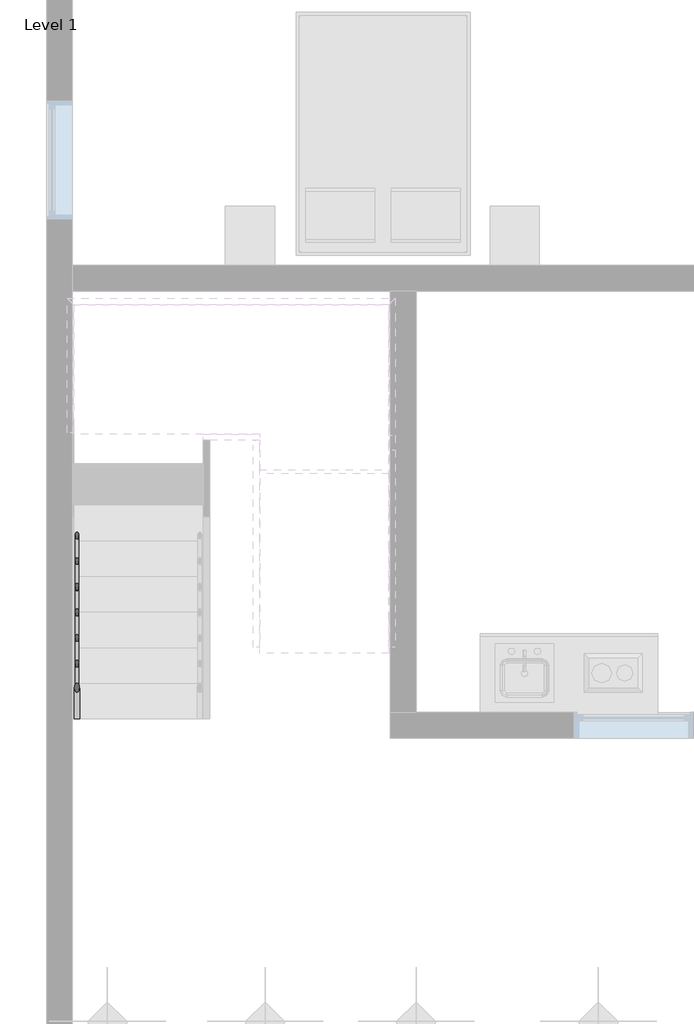
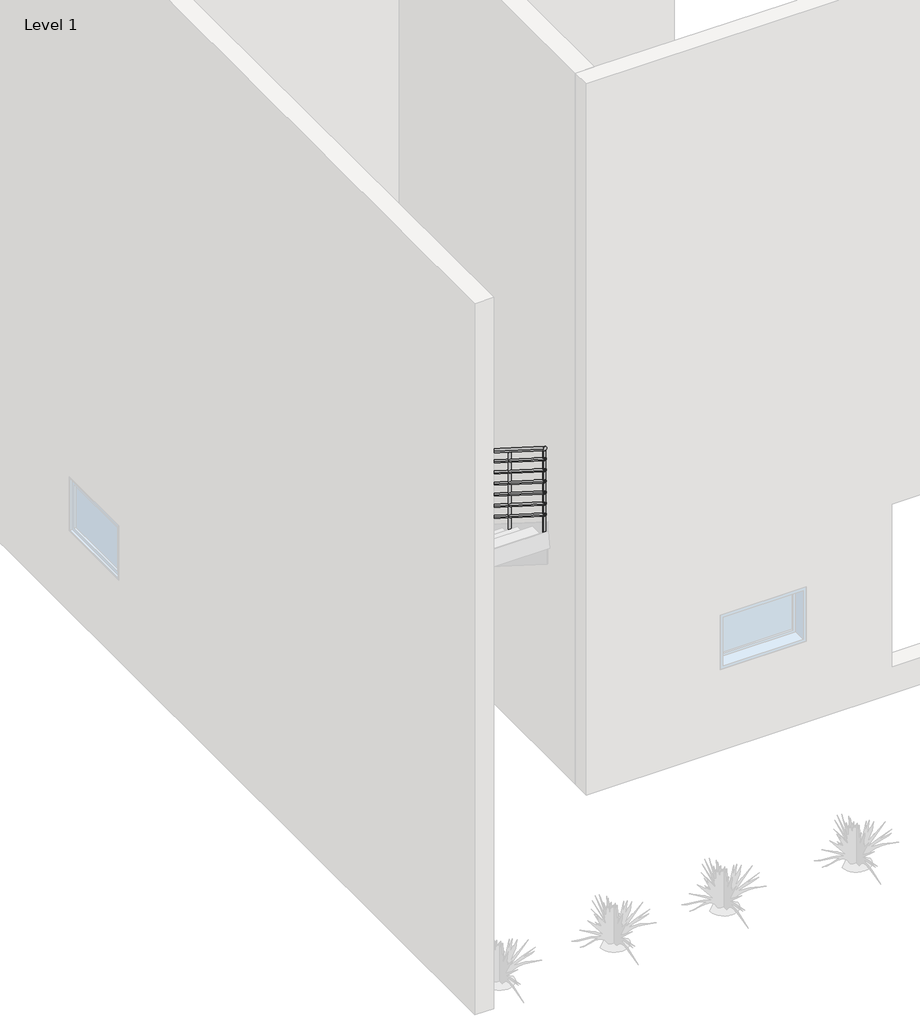
# One storey, part 3 of 4: 1 railing.
"""IFC4 building model written with IfcOpenShell, lengths in millimetres."""

from ifc_helpers import new_model, si_unit, point, frame, frame_2d, origin, place, context, project, spatial, circle_curve, ellipse_curve, trimmed, segment, composite_curve, outline, extrude, element, save
from ifc_brep_helpers import plane_surface, cylinder_surface, advanced_brep

model = new_model("IFC4")

# Units and contexts
model_context = context("Model", 3, world=origin())
ifc_project = project(units=[si_unit("LENGTHUNIT", "METRE", prefix="MILLI")], contexts=[model_context])

# Site, building, storey
site = spatial("IfcSite", under=ifc_project)
building = spatial("IfcBuilding", under=site)
storey = spatial("IfcBuildingStorey", under=building, Name="Level 1", Elevation=0.0)

# Railing
placement = place(None, origin())
element("IfcRailing", 1, ObjectType="900mm Pipe", at=placement, inside=storey, context=model_context, shape_type="SolidModel", body=[
    advanced_brep(
    [(-11976.7805681, 827.4280728, 1050.2491997), (-12016.7805681, 827.4280728, 1050.2491997), (-11976.7805681, 3033.2215258, 2445.2173913), (-12016.7805681, 3033.2215258, 2445.2173913), (-11976.7805681, 3982.053854, 2445.2173913), (-12016.7805681, 4022.053854, 2445.2173913), (-9630.9547869, 3982.053854, 2445.2173913), (-9590.9547869, 4022.053854, 2445.2173913), (-9630.9547869, 3021.6346198, 2445.2173913), (-9590.9547869, 3021.6346198, 2445.2173913), (-9630.9547869, 1377.4280728, 3485.0318084), (-9590.9547869, 1377.4280728, 3485.0318084)],
    [
        (0, 1, ellipse_curve(frame((-11996.7805681, 827.4280728, 1050.2491997), z_axis=(0.0, -1.0, 0.0), x_axis=(0.0, 0.0, -1.0)), 23.6638438, 20.0)),
        (1, 0, ellipse_curve(frame((-11996.7805681, 827.4280728, 1050.2491997), z_axis=(0.0, -1.0, 0.0), x_axis=(0.0, 0.0, -1.0)), 23.6638438, 20.0)),
        (0, 2),
        (2, 3, ellipse_curve(frame((-11996.7805681, 3033.2215258, 2445.2173913), z_axis=(0.0, -0.9605132043335073, -0.2782344053149755), x_axis=(0.0, 0.27823440531497534, -0.9605132043335074)), 20.822202, 20.0)),
        (3, 1),
        (3, 2, ellipse_curve(frame((-11996.7805681, 3033.2215258, 2445.2173913), z_axis=(0.0, -0.9605132043335073, -0.2782344053149755), x_axis=(0.0, 0.27823440531497534, -0.9605132043335074)), 20.822202, 20.0)),
        (2, 4),
        (4, 5, ellipse_curve(frame((-11996.7805681, 4002.053854, 2445.2173913), z_axis=(-0.7071067811865475, -0.7071067811865475, 0.0), x_axis=(0.7071067811865474, -0.7071067811865476, 0.0)), 28.2842712, 20.0)),
        (5, 3),
        (5, 4, ellipse_curve(frame((-11996.7805681, 4002.053854, 2445.2173913), z_axis=(-0.7071067811865475, -0.7071067811865475, 0.0), x_axis=(0.7071067811865474, -0.7071067811865476, 0.0)), 28.2842712, 20.0)),
        (4, 6),
        (6, 7, ellipse_curve(frame((-9610.9547869, 4002.053854, 2445.2173913), z_axis=(-0.7071067811865475, 0.7071067811865475, 0.0), x_axis=(-0.7071067811865476, -0.7071067811865474, 0.0)), 28.2842712, 20.0)),
        (7, 5),
        (7, 6, ellipse_curve(frame((-9610.9547869, 4002.053854, 2445.2173913), z_axis=(-0.7071067811865475, 0.7071067811865475, 0.0), x_axis=(-0.7071067811865476, -0.7071067811865474, 0.0)), 28.2842712, 20.0)),
        (6, 8),
        (8, 9, ellipse_curve(frame((-9610.9547869, 3021.6346198, 2445.2173913), z_axis=(0.0, 0.9605132043335073, -0.27823440531497534), x_axis=(0.0, 0.27823440531497595, 0.9605132043335072)), 20.822202, 20.0)),
        (9, 7),
        (9, 8, ellipse_curve(frame((-9610.9547869, 3021.6346198, 2445.2173913), z_axis=(0.0, 0.9605132043335073, -0.27823440531497534), x_axis=(0.0, 0.27823440531497595, 0.9605132043335072)), 20.822202, 20.0)),
        (10, 11, ellipse_curve(frame((-9610.9547869, 1377.4280728, 3485.0318084), z_axis=(0.0, -1.0, 0.0), x_axis=(0.0, 0.0, -1.0)), 23.6638438, 20.0)),
        (11, 10, ellipse_curve(frame((-9610.9547869, 1377.4280728, 3485.0318084), z_axis=(0.0, -1.0, 0.0), x_axis=(0.0, 0.0, -1.0)), 23.6638438, 20.0)),
        (8, 10),
        (11, 9),
    ],
    [
        plane_surface(frame((-11996.7805681, 827.4280728, 1073.9130435), z_axis=(0.0, -1.0, 0.0), x_axis=(0.0, 0.0, 1.0))),
        cylinder_surface(frame((-11996.7805681, 838.1179856, 1057.0096189), z_axis=(0.0, -0.845171231398044, -0.53449564040983), x_axis=(-1.0, 0.0, 0.0)), 20.0),
        cylinder_surface(frame((-11996.7805681, 3027.4280728, 2445.2173913), z_axis=(0.0, -1.0, 0.0), x_axis=(-1.0, 0.0, 0.0)), 20.0),
        cylinder_surface(frame((-11996.7805681, 4002.053854, 2445.2173913), z_axis=(-1.0, 0.0, 0.0), x_axis=(0.0, 1.0, 0.0)), 20.0),
        cylinder_surface(frame((-9610.9547869, 4002.053854, 2445.2173913), z_axis=(0.0, 1.0, 0.0), x_axis=(1.0, 0.0, 0.0)), 20.0),
        plane_surface(frame((-9610.9547869, 1377.4280728, 3508.6956522), z_axis=(0.0, -1.0, 0.0), x_axis=(0.0, 0.0, -1.0))),
        cylinder_surface(frame((-9610.9547869, 3016.73816, 2448.3139667), z_axis=(0.0, 0.845171231398044, -0.5344956404098297), x_axis=(1.0, 0.0, 0.0)), 20.0),
    ],
    [
        (0, [[1, 2]]),
        (1, [[-1, 3, 4, 5]]),
        (1, [[-2, -5, 6, -3]]),
        (2, [[-4, 7, 8, 9]]),
        (2, [[-6, -9, 10, -7]]),
        (3, [[-8, 11, 12, 13]]),
        (3, [[-10, -13, 14, -11]]),
        (4, [[-12, 15, 16, 17]]),
        (4, [[-14, -17, 18, -15]]),
        (5, [[19, 20]]),
        (6, [[-16, 21, -20, 22]]),
        (6, [[-18, -22, -19, -21]]),
    ],
),
    advanced_brep(
    [(-11981.7805681, 827.4280728, 931.1651606), (-12011.7805681, 827.4280728, 931.1651606), (-11981.7805681, 3031.7731625, 2325.2173913), (-12011.7805681, 3031.7731625, 2325.2173913), (-11981.7805681, 3987.053854, 2325.2173913), (-12011.7805681, 4017.053854, 2325.2173913), (-9625.9547869, 3987.053854, 2325.2173913), (-9595.9547869, 4017.053854, 2325.2173913), (-9625.9547869, 3023.082983, 2325.2173913), (-9595.9547869, 3023.082983, 2325.2173913), (-9625.9547869, 1377.4280728, 3365.9477693), (-9595.9547869, 1377.4280728, 3365.9477693)],
    [
        (0, 1, ellipse_curve(frame((-11996.7805681, 827.4280728, 931.1651606), z_axis=(0.0, -1.0, 0.0), x_axis=(0.0, 0.0, -1.0)), 17.7478828, 15.0)),
        (1, 0, ellipse_curve(frame((-11996.7805681, 827.4280728, 931.1651606), z_axis=(0.0, -1.0, 0.0), x_axis=(0.0, 0.0, -1.0)), 17.7478828, 15.0)),
        (0, 2),
        (2, 3, ellipse_curve(frame((-11996.7805681, 3031.7731625, 2325.2173913), z_axis=(0.0, -0.9605132043335073, -0.2782344053149755), x_axis=(0.0, 0.27823440531497534, -0.9605132043335074)), 15.6166515, 15.0)),
        (3, 1),
        (3, 2, ellipse_curve(frame((-11996.7805681, 3031.7731625, 2325.2173913), z_axis=(0.0, -0.9605132043335073, -0.2782344053149755), x_axis=(0.0, 0.27823440531497534, -0.9605132043335074)), 15.6166515, 15.0)),
        (2, 4),
        (4, 5, ellipse_curve(frame((-11996.7805681, 4002.053854, 2325.2173913), z_axis=(-0.7071067811865475, -0.7071067811865475, 0.0), x_axis=(0.7071067811865474, -0.7071067811865476, 0.0)), 21.2132034, 15.0)),
        (5, 3),
        (5, 4, ellipse_curve(frame((-11996.7805681, 4002.053854, 2325.2173913), z_axis=(-0.7071067811865475, -0.7071067811865475, 0.0), x_axis=(0.7071067811865474, -0.7071067811865476, 0.0)), 21.2132034, 15.0)),
        (4, 6),
        (6, 7, ellipse_curve(frame((-9610.9547869, 4002.053854, 2325.2173913), z_axis=(-0.7071067811865475, 0.7071067811865475, 0.0), x_axis=(-0.7071067811865476, -0.7071067811865474, 0.0)), 21.2132034, 15.0)),
        (7, 5),
        (7, 6, ellipse_curve(frame((-9610.9547869, 4002.053854, 2325.2173913), z_axis=(-0.7071067811865475, 0.7071067811865475, 0.0), x_axis=(-0.7071067811865476, -0.7071067811865474, 0.0)), 21.2132034, 15.0)),
        (6, 8),
        (8, 9, ellipse_curve(frame((-9610.9547869, 3023.082983, 2325.2173913), z_axis=(0.0, 0.9605132043335073, -0.27823440531497534), x_axis=(0.0, 0.27823440531497595, 0.9605132043335072)), 15.6166515, 15.0)),
        (9, 7),
        (9, 8, ellipse_curve(frame((-9610.9547869, 3023.082983, 2325.2173913), z_axis=(0.0, 0.9605132043335073, -0.27823440531497534), x_axis=(0.0, 0.27823440531497595, 0.9605132043335072)), 15.6166515, 15.0)),
        (10, 11, ellipse_curve(frame((-9610.9547869, 1377.4280728, 3365.9477693), z_axis=(0.0, -1.0, 0.0), x_axis=(0.0, 0.0, -1.0)), 17.7478828, 15.0)),
        (11, 10, ellipse_curve(frame((-9610.9547869, 1377.4280728, 3365.9477693), z_axis=(0.0, -1.0, 0.0), x_axis=(0.0, 0.0, -1.0)), 17.7478828, 15.0)),
        (8, 10),
        (11, 9),
    ],
    [
        plane_surface(frame((-11996.7805681, 827.4280728, 948.9130435), z_axis=(0.0, -1.0, 0.0), x_axis=(0.0, 0.0, 1.0))),
        cylinder_surface(frame((-11996.7805681, 835.4455074, 936.235475), z_axis=(0.0, -0.845171231398044, -0.53449564040983), x_axis=(-1.0, 0.0, 0.0)), 15.0),
        cylinder_surface(frame((-11996.7805681, 3027.4280728, 2325.2173913), z_axis=(0.0, -1.0, 0.0), x_axis=(-1.0, 0.0, 0.0)), 15.0),
        cylinder_surface(frame((-11996.7805681, 4002.053854, 2325.2173913), z_axis=(-1.0, 0.0, 0.0), x_axis=(0.0, 1.0, 0.0)), 15.0),
        cylinder_surface(frame((-9610.9547869, 4002.053854, 2325.2173913), z_axis=(0.0, 1.0, 0.0), x_axis=(1.0, 0.0, 0.0)), 15.0),
        plane_surface(frame((-9610.9547869, 1377.4280728, 3383.6956522), z_axis=(0.0, -1.0, 0.0), x_axis=(0.0, 0.0, -1.0))),
        cylinder_surface(frame((-9610.9547869, 3019.4106382, 2327.5398228), z_axis=(0.0, 0.8451712313980441, -0.5344956404098297), x_axis=(1.0, 0.0, 0.0)), 15.0),
    ],
    [
        (0, [[1, 2]]),
        (1, [[-1, 3, 4, 5]]),
        (1, [[-2, -5, 6, -3]]),
        (2, [[-4, 7, 8, 9]]),
        (2, [[-6, -9, 10, -7]]),
        (3, [[-8, 11, 12, 13]]),
        (3, [[-10, -13, 14, -11]]),
        (4, [[-12, 15, 16, 17]]),
        (4, [[-14, -17, 18, -15]]),
        (5, [[19, 20]]),
        (6, [[-16, 21, -20, 22]]),
        (6, [[-18, -22, -19, -21]]),
    ],
),
    advanced_brep(
    [(-11981.7805681, 827.4280728, 806.1651606), (-12011.7805681, 827.4280728, 806.1651606), (-11981.7805681, 3031.7731625, 2200.2173913), (-12011.7805681, 3031.7731625, 2200.2173913), (-11981.7805681, 3987.053854, 2200.2173913), (-12011.7805681, 4017.053854, 2200.2173913), (-9625.9547869, 3987.053854, 2200.2173913), (-9595.9547869, 4017.053854, 2200.2173913), (-9625.9547869, 3023.082983, 2200.2173913), (-9595.9547869, 3023.082983, 2200.2173913), (-9625.9547869, 1377.4280728, 3240.9477693), (-9595.9547869, 1377.4280728, 3240.9477693)],
    [
        (0, 1, ellipse_curve(frame((-11996.7805681, 827.4280728, 806.1651606), z_axis=(0.0, -1.0, 0.0), x_axis=(0.0, 0.0, -1.0)), 17.7478828, 15.0)),
        (1, 0, ellipse_curve(frame((-11996.7805681, 827.4280728, 806.1651606), z_axis=(0.0, -1.0, 0.0), x_axis=(0.0, 0.0, -1.0)), 17.7478828, 15.0)),
        (0, 2),
        (2, 3, ellipse_curve(frame((-11996.7805681, 3031.7731625, 2200.2173913), z_axis=(0.0, -0.9605132043335073, -0.2782344053149755), x_axis=(0.0, 0.27823440531497534, -0.9605132043335074)), 15.6166515, 15.0)),
        (3, 1),
        (3, 2, ellipse_curve(frame((-11996.7805681, 3031.7731625, 2200.2173913), z_axis=(0.0, -0.9605132043335073, -0.2782344053149755), x_axis=(0.0, 0.27823440531497534, -0.9605132043335074)), 15.6166515, 15.0)),
        (2, 4),
        (4, 5, ellipse_curve(frame((-11996.7805681, 4002.053854, 2200.2173913), z_axis=(-0.7071067811865475, -0.7071067811865475, 0.0), x_axis=(0.7071067811865474, -0.7071067811865476, 0.0)), 21.2132034, 15.0)),
        (5, 3),
        (5, 4, ellipse_curve(frame((-11996.7805681, 4002.053854, 2200.2173913), z_axis=(-0.7071067811865475, -0.7071067811865475, 0.0), x_axis=(0.7071067811865474, -0.7071067811865476, 0.0)), 21.2132034, 15.0)),
        (4, 6),
        (6, 7, ellipse_curve(frame((-9610.9547869, 4002.053854, 2200.2173913), z_axis=(-0.7071067811865475, 0.7071067811865475, 0.0), x_axis=(-0.7071067811865476, -0.7071067811865474, 0.0)), 21.2132034, 15.0)),
        (7, 5),
        (7, 6, ellipse_curve(frame((-9610.9547869, 4002.053854, 2200.2173913), z_axis=(-0.7071067811865475, 0.7071067811865475, 0.0), x_axis=(-0.7071067811865476, -0.7071067811865474, 0.0)), 21.2132034, 15.0)),
        (6, 8),
        (8, 9, ellipse_curve(frame((-9610.9547869, 3023.082983, 2200.2173913), z_axis=(0.0, 0.9605132043335073, -0.27823440531497534), x_axis=(0.0, 0.27823440531497595, 0.9605132043335072)), 15.6166515, 15.0)),
        (9, 7),
        (9, 8, ellipse_curve(frame((-9610.9547869, 3023.082983, 2200.2173913), z_axis=(0.0, 0.9605132043335073, -0.27823440531497534), x_axis=(0.0, 0.27823440531497595, 0.9605132043335072)), 15.6166515, 15.0)),
        (10, 11, ellipse_curve(frame((-9610.9547869, 1377.4280728, 3240.9477693), z_axis=(0.0, -1.0, 0.0), x_axis=(0.0, 0.0, -1.0)), 17.7478828, 15.0)),
        (11, 10, ellipse_curve(frame((-9610.9547869, 1377.4280728, 3240.9477693), z_axis=(0.0, -1.0, 0.0), x_axis=(0.0, 0.0, -1.0)), 17.7478828, 15.0)),
        (8, 10),
        (11, 9),
    ],
    [
        plane_surface(frame((-11996.7805681, 827.4280728, 823.9130435), z_axis=(0.0, -1.0, 0.0), x_axis=(0.0, 0.0, 1.0))),
        cylinder_surface(frame((-11996.7805681, 835.4455074, 811.235475), z_axis=(0.0, -0.845171231398044, -0.53449564040983), x_axis=(-1.0, 0.0, 0.0)), 15.0),
        cylinder_surface(frame((-11996.7805681, 3027.4280728, 2200.2173913), z_axis=(0.0, -1.0, 0.0), x_axis=(-1.0, 0.0, 0.0)), 15.0),
        cylinder_surface(frame((-11996.7805681, 4002.053854, 2200.2173913), z_axis=(-1.0, 0.0, 0.0), x_axis=(0.0, 1.0, 0.0)), 15.0),
        cylinder_surface(frame((-9610.9547869, 4002.053854, 2200.2173913), z_axis=(0.0, 1.0, 0.0), x_axis=(1.0, 0.0, 0.0)), 15.0),
        plane_surface(frame((-9610.9547869, 1377.4280728, 3258.6956522), z_axis=(0.0, -1.0, 0.0), x_axis=(0.0, 0.0, -1.0))),
        cylinder_surface(frame((-9610.9547869, 3019.4106382, 2202.5398228), z_axis=(0.0, 0.845171231398044, -0.5344956404098297), x_axis=(1.0, 0.0, 0.0)), 15.0),
    ],
    [
        (0, [[1, 2]]),
        (1, [[-1, 3, 4, 5]]),
        (1, [[-2, -5, 6, -3]]),
        (2, [[-4, 7, 8, 9]]),
        (2, [[-6, -9, 10, -7]]),
        (3, [[-8, 11, 12, 13]]),
        (3, [[-10, -13, 14, -11]]),
        (4, [[-12, 15, 16, 17]]),
        (4, [[-14, -17, 18, -15]]),
        (5, [[19, 20]]),
        (6, [[-16, 21, -20, 22]]),
        (6, [[-18, -22, -19, -21]]),
    ],
),
    advanced_brep(
    [(-11981.7805681, 827.4280728, 681.1651606), (-12011.7805681, 827.4280728, 681.1651606), (-11981.7805681, 3031.7731625, 2075.2173913), (-12011.7805681, 3031.7731625, 2075.2173913), (-11981.7805681, 3987.053854, 2075.2173913), (-12011.7805681, 4017.053854, 2075.2173913), (-9625.9547869, 3987.053854, 2075.2173913), (-9595.9547869, 4017.053854, 2075.2173913), (-9625.9547869, 3023.082983, 2075.2173913), (-9595.9547869, 3023.082983, 2075.2173913), (-9625.9547869, 1377.4280728, 3115.9477693), (-9595.9547869, 1377.4280728, 3115.9477693)],
    [
        (0, 1, ellipse_curve(frame((-11996.7805681, 827.4280728, 681.1651606), z_axis=(0.0, -1.0, 0.0), x_axis=(0.0, 0.0, -1.0)), 17.7478828, 15.0)),
        (1, 0, ellipse_curve(frame((-11996.7805681, 827.4280728, 681.1651606), z_axis=(0.0, -1.0, 0.0), x_axis=(0.0, 0.0, -1.0)), 17.7478828, 15.0)),
        (0, 2),
        (2, 3, ellipse_curve(frame((-11996.7805681, 3031.7731625, 2075.2173913), z_axis=(0.0, -0.9605132043335073, -0.2782344053149755), x_axis=(0.0, 0.27823440531497534, -0.9605132043335074)), 15.6166515, 15.0)),
        (3, 1),
        (3, 2, ellipse_curve(frame((-11996.7805681, 3031.7731625, 2075.2173913), z_axis=(0.0, -0.9605132043335073, -0.2782344053149755), x_axis=(0.0, 0.27823440531497534, -0.9605132043335074)), 15.6166515, 15.0)),
        (2, 4),
        (4, 5, ellipse_curve(frame((-11996.7805681, 4002.053854, 2075.2173913), z_axis=(-0.7071067811865475, -0.7071067811865475, 0.0), x_axis=(0.7071067811865474, -0.7071067811865476, 0.0)), 21.2132034, 15.0)),
        (5, 3),
        (5, 4, ellipse_curve(frame((-11996.7805681, 4002.053854, 2075.2173913), z_axis=(-0.7071067811865475, -0.7071067811865475, 0.0), x_axis=(0.7071067811865474, -0.7071067811865476, 0.0)), 21.2132034, 15.0)),
        (4, 6),
        (6, 7, ellipse_curve(frame((-9610.9547869, 4002.053854, 2075.2173913), z_axis=(-0.7071067811865475, 0.7071067811865475, 0.0), x_axis=(-0.7071067811865476, -0.7071067811865474, 0.0)), 21.2132034, 15.0)),
        (7, 5),
        (7, 6, ellipse_curve(frame((-9610.9547869, 4002.053854, 2075.2173913), z_axis=(-0.7071067811865475, 0.7071067811865475, 0.0), x_axis=(-0.7071067811865476, -0.7071067811865474, 0.0)), 21.2132034, 15.0)),
        (6, 8),
        (8, 9, ellipse_curve(frame((-9610.9547869, 3023.082983, 2075.2173913), z_axis=(0.0, 0.9605132043335073, -0.2782344053149754), x_axis=(0.0, 0.2782344053149759, 0.9605132043335072)), 15.6166515, 15.0)),
        (9, 7),
        (9, 8, ellipse_curve(frame((-9610.9547869, 3023.082983, 2075.2173913), z_axis=(0.0, 0.9605132043335073, -0.2782344053149754), x_axis=(0.0, 0.2782344053149759, 0.9605132043335072)), 15.6166515, 15.0)),
        (10, 11, ellipse_curve(frame((-9610.9547869, 1377.4280728, 3115.9477693), z_axis=(0.0, -1.0, 0.0), x_axis=(0.0, 0.0, -1.0)), 17.7478828, 15.0)),
        (11, 10, ellipse_curve(frame((-9610.9547869, 1377.4280728, 3115.9477693), z_axis=(0.0, -1.0, 0.0), x_axis=(0.0, 0.0, -1.0)), 17.7478828, 15.0)),
        (8, 10),
        (11, 9),
    ],
    [
        plane_surface(frame((-11996.7805681, 827.4280728, 698.9130435), z_axis=(0.0, -1.0, 0.0), x_axis=(0.0, 0.0, 1.0))),
        cylinder_surface(frame((-11996.7805681, 835.4455074, 686.235475), z_axis=(0.0, -0.845171231398044, -0.53449564040983), x_axis=(-1.0, 0.0, 0.0)), 15.0),
        cylinder_surface(frame((-11996.7805681, 3027.4280728, 2075.2173913), z_axis=(0.0, -1.0, 0.0), x_axis=(-1.0, 0.0, 0.0)), 15.0),
        cylinder_surface(frame((-11996.7805681, 4002.053854, 2075.2173913), z_axis=(-1.0, 0.0, 0.0), x_axis=(0.0, 1.0, 0.0)), 15.0),
        cylinder_surface(frame((-9610.9547869, 4002.053854, 2075.2173913), z_axis=(0.0, 1.0, 0.0), x_axis=(1.0, 0.0, 0.0)), 15.0),
        plane_surface(frame((-9610.9547869, 1377.4280728, 3133.6956522), z_axis=(0.0, -1.0, 0.0), x_axis=(0.0, 0.0, -1.0))),
        cylinder_surface(frame((-9610.9547869, 3019.4106382, 2077.5398228), z_axis=(0.0, 0.845171231398044, -0.5344956404098298), x_axis=(1.0, 0.0, 0.0)), 15.0),
    ],
    [
        (0, [[1, 2]]),
        (1, [[-1, 3, 4, 5]]),
        (1, [[-2, -5, 6, -3]]),
        (2, [[-4, 7, 8, 9]]),
        (2, [[-6, -9, 10, -7]]),
        (3, [[-8, 11, 12, 13]]),
        (3, [[-10, -13, 14, -11]]),
        (4, [[-12, 15, 16, 17]]),
        (4, [[-14, -17, 18, -15]]),
        (5, [[19, 20]]),
        (6, [[-16, 21, -20, 22]]),
        (6, [[-18, -22, -19, -21]]),
    ],
),
    advanced_brep(
    [(-11981.7805681, 827.4280728, 556.1651606), (-12011.7805681, 827.4280728, 556.1651606), (-11981.7805681, 3031.7731625, 1950.2173913), (-12011.7805681, 3031.7731625, 1950.2173913), (-11981.7805681, 3987.053854, 1950.2173913), (-12011.7805681, 4017.053854, 1950.2173913), (-9625.9547869, 3987.053854, 1950.2173913), (-9595.9547869, 4017.053854, 1950.2173913), (-9625.9547869, 3023.082983, 1950.2173913), (-9595.9547869, 3023.082983, 1950.2173913), (-9625.9547869, 1377.4280728, 2990.9477693), (-9595.9547869, 1377.4280728, 2990.9477693)],
    [
        (0, 1, ellipse_curve(frame((-11996.7805681, 827.4280728, 556.1651606), z_axis=(0.0, -1.0, 0.0), x_axis=(0.0, 0.0, -1.0)), 17.7478828, 15.0)),
        (1, 0, ellipse_curve(frame((-11996.7805681, 827.4280728, 556.1651606), z_axis=(0.0, -1.0, 0.0), x_axis=(0.0, 0.0, -1.0)), 17.7478828, 15.0)),
        (0, 2),
        (2, 3, ellipse_curve(frame((-11996.7805681, 3031.7731625, 1950.2173913), z_axis=(0.0, -0.9605132043335073, -0.2782344053149755), x_axis=(0.0, 0.27823440531497534, -0.9605132043335074)), 15.6166515, 15.0)),
        (3, 1),
        (3, 2, ellipse_curve(frame((-11996.7805681, 3031.7731625, 1950.2173913), z_axis=(0.0, -0.9605132043335073, -0.2782344053149755), x_axis=(0.0, 0.27823440531497534, -0.9605132043335074)), 15.6166515, 15.0)),
        (2, 4),
        (4, 5, ellipse_curve(frame((-11996.7805681, 4002.053854, 1950.2173913), z_axis=(-0.7071067811865475, -0.7071067811865475, 0.0), x_axis=(0.7071067811865474, -0.7071067811865476, 0.0)), 21.2132034, 15.0)),
        (5, 3),
        (5, 4, ellipse_curve(frame((-11996.7805681, 4002.053854, 1950.2173913), z_axis=(-0.7071067811865475, -0.7071067811865475, 0.0), x_axis=(0.7071067811865474, -0.7071067811865476, 0.0)), 21.2132034, 15.0)),
        (4, 6),
        (6, 7, ellipse_curve(frame((-9610.9547869, 4002.053854, 1950.2173913), z_axis=(-0.7071067811865475, 0.7071067811865475, 0.0), x_axis=(-0.7071067811865476, -0.7071067811865474, 0.0)), 21.2132034, 15.0)),
        (7, 5),
        (7, 6, ellipse_curve(frame((-9610.9547869, 4002.053854, 1950.2173913), z_axis=(-0.7071067811865475, 0.7071067811865475, 0.0), x_axis=(-0.7071067811865476, -0.7071067811865474, 0.0)), 21.2132034, 15.0)),
        (6, 8),
        (8, 9, ellipse_curve(frame((-9610.9547869, 3023.082983, 1950.2173913), z_axis=(0.0, 0.9605132043335073, -0.27823440531497534), x_axis=(0.0, 0.27823440531497595, 0.9605132043335072)), 15.6166515, 15.0)),
        (9, 7),
        (9, 8, ellipse_curve(frame((-9610.9547869, 3023.082983, 1950.2173913), z_axis=(0.0, 0.9605132043335073, -0.27823440531497534), x_axis=(0.0, 0.27823440531497595, 0.9605132043335072)), 15.6166515, 15.0)),
        (10, 11, ellipse_curve(frame((-9610.9547869, 1377.4280728, 2990.9477693), z_axis=(0.0, -1.0, 0.0), x_axis=(0.0, 0.0, -1.0)), 17.7478828, 15.0)),
        (11, 10, ellipse_curve(frame((-9610.9547869, 1377.4280728, 2990.9477693), z_axis=(0.0, -1.0, 0.0), x_axis=(0.0, 0.0, -1.0)), 17.7478828, 15.0)),
        (8, 10),
        (11, 9),
    ],
    [
        plane_surface(frame((-11996.7805681, 827.4280728, 573.9130435), z_axis=(0.0, -1.0, 0.0), x_axis=(0.0, 0.0, 1.0))),
        cylinder_surface(frame((-11996.7805681, 835.4455074, 561.235475), z_axis=(0.0, -0.845171231398044, -0.53449564040983), x_axis=(-1.0, 0.0, 0.0)), 15.0),
        cylinder_surface(frame((-11996.7805681, 3027.4280728, 1950.2173913), z_axis=(0.0, -1.0, 0.0), x_axis=(-1.0, 0.0, 0.0)), 15.0),
        cylinder_surface(frame((-11996.7805681, 4002.053854, 1950.2173913), z_axis=(-1.0, 0.0, 0.0), x_axis=(0.0, 1.0, 0.0)), 15.0),
        cylinder_surface(frame((-9610.9547869, 4002.053854, 1950.2173913), z_axis=(0.0, 1.0, 0.0), x_axis=(1.0, 0.0, 0.0)), 15.0),
        plane_surface(frame((-9610.9547869, 1377.4280728, 3008.6956522), z_axis=(0.0, -1.0, 0.0), x_axis=(0.0, 0.0, -1.0))),
        cylinder_surface(frame((-9610.9547869, 3019.4106382, 1952.5398228), z_axis=(0.0, 0.845171231398044, -0.5344956404098297), x_axis=(1.0, 0.0, 0.0)), 15.0),
    ],
    [
        (0, [[1, 2]]),
        (1, [[-1, 3, 4, 5]]),
        (1, [[-2, -5, 6, -3]]),
        (2, [[-4, 7, 8, 9]]),
        (2, [[-6, -9, 10, -7]]),
        (3, [[-8, 11, 12, 13]]),
        (3, [[-10, -13, 14, -11]]),
        (4, [[-12, 15, 16, 17]]),
        (4, [[-14, -17, 18, -15]]),
        (5, [[19, 20]]),
        (6, [[-16, 21, -20, 22]]),
        (6, [[-18, -22, -19, -21]]),
    ],
),
    advanced_brep(
    [(-11981.7805681, 827.4280728, 431.1651606), (-12011.7805681, 827.4280728, 431.1651606), (-11981.7805681, 3031.7731625, 1825.2173913), (-12011.7805681, 3031.7731625, 1825.2173913), (-11981.7805681, 3987.053854, 1825.2173913), (-12011.7805681, 4017.053854, 1825.2173913), (-9625.9547869, 3987.053854, 1825.2173913), (-9595.9547869, 4017.053854, 1825.2173913), (-9625.9547869, 3023.082983, 1825.2173913), (-9595.9547869, 3023.082983, 1825.2173913), (-9625.9547869, 1377.4280728, 2865.9477693), (-9595.9547869, 1377.4280728, 2865.9477693)],
    [
        (0, 1, ellipse_curve(frame((-11996.7805681, 827.4280728, 431.1651606), z_axis=(0.0, -1.0, 0.0), x_axis=(0.0, 0.0, -1.0)), 17.7478828, 15.0)),
        (1, 0, ellipse_curve(frame((-11996.7805681, 827.4280728, 431.1651606), z_axis=(0.0, -1.0, 0.0), x_axis=(0.0, 0.0, -1.0)), 17.7478828, 15.0)),
        (0, 2),
        (2, 3, ellipse_curve(frame((-11996.7805681, 3031.7731625, 1825.2173913), z_axis=(0.0, -0.9605132043335073, -0.2782344053149755), x_axis=(0.0, 0.27823440531497534, -0.9605132043335074)), 15.6166515, 15.0)),
        (3, 1),
        (3, 2, ellipse_curve(frame((-11996.7805681, 3031.7731625, 1825.2173913), z_axis=(0.0, -0.9605132043335073, -0.2782344053149755), x_axis=(0.0, 0.27823440531497534, -0.9605132043335074)), 15.6166515, 15.0)),
        (2, 4),
        (4, 5, ellipse_curve(frame((-11996.7805681, 4002.053854, 1825.2173913), z_axis=(-0.7071067811865475, -0.7071067811865475, 0.0), x_axis=(0.7071067811865474, -0.7071067811865476, 0.0)), 21.2132034, 15.0)),
        (5, 3),
        (5, 4, ellipse_curve(frame((-11996.7805681, 4002.053854, 1825.2173913), z_axis=(-0.7071067811865475, -0.7071067811865475, 0.0), x_axis=(0.7071067811865474, -0.7071067811865476, 0.0)), 21.2132034, 15.0)),
        (4, 6),
        (6, 7, ellipse_curve(frame((-9610.9547869, 4002.053854, 1825.2173913), z_axis=(-0.7071067811865475, 0.7071067811865475, 0.0), x_axis=(-0.7071067811865476, -0.7071067811865474, 0.0)), 21.2132034, 15.0)),
        (7, 5),
        (7, 6, ellipse_curve(frame((-9610.9547869, 4002.053854, 1825.2173913), z_axis=(-0.7071067811865475, 0.7071067811865475, 0.0), x_axis=(-0.7071067811865476, -0.7071067811865474, 0.0)), 21.2132034, 15.0)),
        (6, 8),
        (8, 9, ellipse_curve(frame((-9610.9547869, 3023.082983, 1825.2173913), z_axis=(0.0, 0.9605132043335073, -0.27823440531497534), x_axis=(0.0, 0.27823440531497595, 0.9605132043335072)), 15.6166515, 15.0)),
        (9, 7),
        (9, 8, ellipse_curve(frame((-9610.9547869, 3023.082983, 1825.2173913), z_axis=(0.0, 0.9605132043335073, -0.27823440531497534), x_axis=(0.0, 0.27823440531497595, 0.9605132043335072)), 15.6166515, 15.0)),
        (10, 11, ellipse_curve(frame((-9610.9547869, 1377.4280728, 2865.9477693), z_axis=(0.0, -1.0, 0.0), x_axis=(0.0, 0.0, -1.0)), 17.7478828, 15.0)),
        (11, 10, ellipse_curve(frame((-9610.9547869, 1377.4280728, 2865.9477693), z_axis=(0.0, -1.0, 0.0), x_axis=(0.0, 0.0, -1.0)), 17.7478828, 15.0)),
        (8, 10),
        (11, 9),
    ],
    [
        plane_surface(frame((-11996.7805681, 827.4280728, 448.9130435), z_axis=(0.0, -1.0, 0.0), x_axis=(0.0, 0.0, 1.0))),
        cylinder_surface(frame((-11996.7805681, 835.4455074, 436.235475), z_axis=(0.0, -0.845171231398044, -0.53449564040983), x_axis=(-1.0, 0.0, 0.0)), 15.0),
        cylinder_surface(frame((-11996.7805681, 3027.4280728, 1825.2173913), z_axis=(0.0, -1.0, 0.0), x_axis=(-1.0, 0.0, 0.0)), 15.0),
        cylinder_surface(frame((-11996.7805681, 4002.053854, 1825.2173913), z_axis=(-1.0, 0.0, 0.0), x_axis=(0.0, 1.0, 0.0)), 15.0),
        cylinder_surface(frame((-9610.9547869, 4002.053854, 1825.2173913), z_axis=(0.0, 1.0, 0.0), x_axis=(1.0, 0.0, 0.0)), 15.0),
        plane_surface(frame((-9610.9547869, 1377.4280728, 2883.6956522), z_axis=(0.0, -1.0, 0.0), x_axis=(0.0, 0.0, -1.0))),
        cylinder_surface(frame((-9610.9547869, 3019.4106382, 1827.5398228), z_axis=(0.0, 0.8451712313980441, -0.5344956404098297), x_axis=(1.0, 0.0, 0.0)), 15.0),
    ],
    [
        (0, [[1, 2]]),
        (1, [[-1, 3, 4, 5]]),
        (1, [[-2, -5, 6, -3]]),
        (2, [[-4, 7, 8, 9]]),
        (2, [[-6, -9, 10, -7]]),
        (3, [[-8, 11, 12, 13]]),
        (3, [[-10, -13, 14, -11]]),
        (4, [[-12, 15, 16, 17]]),
        (4, [[-14, -17, 18, -15]]),
        (5, [[19, 20]]),
        (6, [[-16, 21, -20, 22]]),
        (6, [[-18, -22, -19, -21]]),
    ],
),
    advanced_brep(
    [(-11981.7805681, 827.4280728, 306.1651606), (-12011.7805681, 827.4280728, 306.1651606), (-11981.7805681, 3031.7731625, 1700.2173913), (-12011.7805681, 3031.7731625, 1700.2173913), (-11981.7805681, 3987.053854, 1700.2173913), (-12011.7805681, 4017.053854, 1700.2173913), (-9625.9547869, 3987.053854, 1700.2173913), (-9595.9547869, 4017.053854, 1700.2173913), (-9625.9547869, 3023.082983, 1700.2173913), (-9595.9547869, 3023.082983, 1700.2173913), (-9625.9547869, 1377.4280728, 2740.9477693), (-9595.9547869, 1377.4280728, 2740.9477693)],
    [
        (0, 1, ellipse_curve(frame((-11996.7805681, 827.4280728, 306.1651606), z_axis=(0.0, -1.0, 0.0), x_axis=(0.0, 0.0, -1.0)), 17.7478828, 15.0)),
        (1, 0, ellipse_curve(frame((-11996.7805681, 827.4280728, 306.1651606), z_axis=(0.0, -1.0, 0.0), x_axis=(0.0, 0.0, -1.0)), 17.7478828, 15.0)),
        (0, 2),
        (2, 3, ellipse_curve(frame((-11996.7805681, 3031.7731625, 1700.2173913), z_axis=(0.0, -0.9605132043335073, -0.2782344053149755), x_axis=(0.0, 0.27823440531497534, -0.9605132043335074)), 15.6166515, 15.0)),
        (3, 1),
        (3, 2, ellipse_curve(frame((-11996.7805681, 3031.7731625, 1700.2173913), z_axis=(0.0, -0.9605132043335073, -0.2782344053149755), x_axis=(0.0, 0.27823440531497534, -0.9605132043335074)), 15.6166515, 15.0)),
        (2, 4),
        (4, 5, ellipse_curve(frame((-11996.7805681, 4002.053854, 1700.2173913), z_axis=(-0.7071067811865475, -0.7071067811865475, 0.0), x_axis=(0.7071067811865474, -0.7071067811865476, 0.0)), 21.2132034, 15.0)),
        (5, 3),
        (5, 4, ellipse_curve(frame((-11996.7805681, 4002.053854, 1700.2173913), z_axis=(-0.7071067811865475, -0.7071067811865475, 0.0), x_axis=(0.7071067811865474, -0.7071067811865476, 0.0)), 21.2132034, 15.0)),
        (4, 6),
        (6, 7, ellipse_curve(frame((-9610.9547869, 4002.053854, 1700.2173913), z_axis=(-0.7071067811865475, 0.7071067811865475, 0.0), x_axis=(-0.7071067811865476, -0.7071067811865474, 0.0)), 21.2132034, 15.0)),
        (7, 5),
        (7, 6, ellipse_curve(frame((-9610.9547869, 4002.053854, 1700.2173913), z_axis=(-0.7071067811865475, 0.7071067811865475, 0.0), x_axis=(-0.7071067811865476, -0.7071067811865474, 0.0)), 21.2132034, 15.0)),
        (6, 8),
        (8, 9, ellipse_curve(frame((-9610.9547869, 3023.082983, 1700.2173913), z_axis=(0.0, 0.9605132043335073, -0.27823440531497534), x_axis=(0.0, 0.27823440531497595, 0.9605132043335072)), 15.6166515, 15.0)),
        (9, 7),
        (9, 8, ellipse_curve(frame((-9610.9547869, 3023.082983, 1700.2173913), z_axis=(0.0, 0.9605132043335073, -0.27823440531497534), x_axis=(0.0, 0.27823440531497595, 0.9605132043335072)), 15.6166515, 15.0)),
        (10, 11, ellipse_curve(frame((-9610.9547869, 1377.4280728, 2740.9477693), z_axis=(0.0, -1.0, 0.0), x_axis=(0.0, 0.0, -1.0)), 17.7478828, 15.0)),
        (11, 10, ellipse_curve(frame((-9610.9547869, 1377.4280728, 2740.9477693), z_axis=(0.0, -1.0, 0.0), x_axis=(0.0, 0.0, -1.0)), 17.7478828, 15.0)),
        (8, 10),
        (11, 9),
    ],
    [
        plane_surface(frame((-11996.7805681, 827.4280728, 323.9130435), z_axis=(0.0, -1.0, 0.0), x_axis=(0.0, 0.0, 1.0))),
        cylinder_surface(frame((-11996.7805681, 835.4455074, 311.235475), z_axis=(0.0, -0.845171231398044, -0.53449564040983), x_axis=(-1.0, 0.0, 0.0)), 15.0),
        cylinder_surface(frame((-11996.7805681, 3027.4280728, 1700.2173913), z_axis=(0.0, -1.0, 0.0), x_axis=(-1.0, 0.0, 0.0)), 15.0),
        cylinder_surface(frame((-11996.7805681, 4002.053854, 1700.2173913), z_axis=(-1.0, 0.0, 0.0), x_axis=(0.0, 1.0, 0.0)), 15.0),
        cylinder_surface(frame((-9610.9547869, 4002.053854, 1700.2173913), z_axis=(0.0, 1.0, 0.0), x_axis=(1.0, 0.0, 0.0)), 15.0),
        plane_surface(frame((-9610.9547869, 1377.4280728, 2758.6956522), z_axis=(0.0, -1.0, 0.0), x_axis=(0.0, 0.0, -1.0))),
        cylinder_surface(frame((-9610.9547869, 3019.4106382, 1702.5398228), z_axis=(0.0, 0.845171231398044, -0.5344956404098297), x_axis=(1.0, 0.0, 0.0)), 15.0),
    ],
    [
        (0, [[1, 2]]),
        (1, [[-1, 3, 4, 5]]),
        (1, [[-2, -5, 6, -3]]),
        (2, [[-4, 7, 8, 9]]),
        (2, [[-6, -9, 10, -7]]),
        (3, [[-8, 11, 12, 13]]),
        (3, [[-10, -13, 14, -11]]),
        (4, [[-12, 15, 16, 17]]),
        (4, [[-14, -17, 18, -15]]),
        (5, [[19, 20]]),
        (6, [[-16, 21, -20, 22]]),
        (6, [[-18, -22, -19, -21]]),
    ],
),
    advanced_brep(
    [(-9598.4547869, 2027.4280728, 3050.3007709), (-9623.4547869, 2027.4280728, 3050.3007709), (-9623.4547869, 2027.4280728, 2086.9565217), (-9598.4547869, 2027.4280728, 2086.9565217)],
    [
        (0, 1, ellipse_curve(frame((-9610.9547869, 2027.4280728, 3050.3007709), z_axis=(0.0, -0.5344956404098286, -0.8451712313980447), x_axis=(0.0, -0.8451712313980447, 0.5344956404098286)), 14.7899024, 12.5)),
        (1, 2),
        (2, 3, circle_curve(frame((-9610.9547869, 2027.4280728, 2086.9565217), z_axis=(0.0, 0.0, 1.0), x_axis=(-1.0, 0.0, 0.0)), 12.5)),
        (3, 0),
        (3, 2, circle_curve(frame((-9610.9547869, 2027.4280728, 2086.9565217), z_axis=(0.0, 0.0, 1.0), x_axis=(-1.0, 0.0, 0.0)), 12.5)),
        (1, 0, ellipse_curve(frame((-9610.9547869, 2027.4280728, 3050.3007709), z_axis=(0.0, -0.5344956404098286, -0.8451712313980447), x_axis=(0.0, -0.8451712313980447, 0.5344956404098286)), 14.7899024, 12.5)),
    ],
    [
        cylinder_surface(frame((-9610.9547869, 2027.4280728, 1986.9565217), z_axis=(0.0, 0.0, 1.0), x_axis=(-1.0, 0.0, 0.0)), 12.5),
        plane_surface(frame((-9635.9547869, 2002.4280728, 3066.1110476), z_axis=(0.0, 0.5344956404098286, 0.8451712313980447), x_axis=(1.0, 0.0, 0.0))),
        plane_surface(frame((-9635.9547869, 2052.4280728, 2086.9565217), z_axis=(0.0, 0.0, -1.0), x_axis=(1.0, 0.0, 0.0))),
    ],
    [
        (0, [[1, 2, 3, 4]]),
        (0, [[5, -2, 6, -4]]),
        (1, [[-6, -1]]),
        (2, [[-5, -3]]),
    ],
),
    extrude(outline(composite_curve([segment(trimmed(circle_curve(frame_2d((-9996.7805681, 4002.053854)), 12.5), [point((-9996.7805681, 3989.553854))], [point((-9996.7805681, 4014.553854))], False, "CARTESIAN"), True, "CONTINUOUS"), segment(trimmed(circle_curve(frame_2d((-9996.7805681, 4002.053854)), 12.5), [point((-9996.7805681, 4014.553854))], [point((-9996.7805681, 3989.553854))], False, "CARTESIAN"), True, "CONTINUOUS")], self_intersect=False)), frame((0.0, 0.0, 1565.2173913), z_axis=(0.0, 0.0, 1.0), x_axis=(1.0, 0.0, 0.0)), (0.0, 0.0, 1.0), 860.0),
    extrude(outline(composite_curve([segment(trimmed(circle_curve(frame_2d((-10996.7805681, 4002.053854)), 12.5), [point((-10996.7805681, 3989.553854))], [point((-10996.7805681, 4014.553854))], False, "CARTESIAN"), True, "CONTINUOUS"), segment(trimmed(circle_curve(frame_2d((-10996.7805681, 4002.053854)), 12.5), [point((-10996.7805681, 4014.553854))], [point((-10996.7805681, 3989.553854))], False, "CARTESIAN"), True, "CONTINUOUS")], self_intersect=False)), frame((0.0, 0.0, 1565.2173913), z_axis=(0.0, 0.0, 1.0), x_axis=(1.0, 0.0, 0.0)), (0.0, 0.0, 1.0), 860.0),
    advanced_brep(
    [(-12009.2805681, 2827.4280728, 2291.4074903), (-11984.2805681, 2827.4280728, 2291.4074903), (-11984.2805681, 2827.4280728, 1391.3043478), (-12009.2805681, 2827.4280728, 1391.3043478)],
    [
        (0, 1, ellipse_curve(frame((-11996.7805681, 2827.4280728, 2291.4074903), z_axis=(0.0, 0.5344956404098302, -0.8451712313980437), x_axis=(0.0, 0.8451712313980437, 0.53449564040983)), 14.7899024, 12.5)),
        (1, 2),
        (2, 3, circle_curve(frame((-11996.7805681, 2827.4280728, 1391.3043478), z_axis=(0.0, 0.0, 1.0), x_axis=(1.0, 0.0, 0.0)), 12.5)),
        (3, 0),
        (3, 2, circle_curve(frame((-11996.7805681, 2827.4280728, 1391.3043478), z_axis=(0.0, 0.0, 1.0), x_axis=(1.0, 0.0, 0.0)), 12.5)),
        (1, 0, ellipse_curve(frame((-11996.7805681, 2827.4280728, 2291.4074903), z_axis=(0.0, 0.5344956404098302, -0.8451712313980437), x_axis=(0.0, 0.8451712313980437, 0.53449564040983)), 14.7899024, 12.5)),
    ],
    [
        cylinder_surface(frame((-11996.7805681, 2827.4280728, 1291.3043478), z_axis=(0.0, 0.0, 1.0), x_axis=(1.0, 0.0, 0.0)), 12.5),
        plane_surface(frame((-11971.7805681, 2852.4280728, 2307.217767), z_axis=(0.0, -0.5344956404098302, 0.8451712313980437), x_axis=(-1.0, 0.0, 0.0))),
        plane_surface(frame((-11971.7805681, 2802.4280728, 1391.3043478), z_axis=(0.0, 0.0, -1.0), x_axis=(-1.0, 0.0, 0.0))),
    ],
    [
        (0, [[1, 2, 3, 4]]),
        (0, [[5, -2, 6, -4]]),
        (1, [[-6, -1]]),
        (2, [[-5, -3]]),
    ],
),
    advanced_brep(
    [(-12009.2805681, 1827.4280728, 1658.9964231), (-11984.2805681, 1827.4280728, 1658.9964231), (-11984.2805681, 1827.4280728, 695.6521739), (-12009.2805681, 1827.4280728, 695.6521739)],
    [
        (0, 1, ellipse_curve(frame((-11996.7805681, 1827.4280728, 1658.9964231), z_axis=(0.0, 0.5344956404098286, -0.8451712313980447), x_axis=(0.0, 0.8451712313980447, 0.5344956404098286)), 14.7899024, 12.5)),
        (1, 2),
        (2, 3, circle_curve(frame((-11996.7805681, 1827.4280728, 695.6521739), z_axis=(0.0, 0.0, 1.0), x_axis=(1.0, 0.0, 0.0)), 12.5)),
        (3, 0),
        (3, 2, circle_curve(frame((-11996.7805681, 1827.4280728, 695.6521739), z_axis=(0.0, 0.0, 1.0), x_axis=(1.0, 0.0, 0.0)), 12.5)),
        (1, 0, ellipse_curve(frame((-11996.7805681, 1827.4280728, 1658.9964231), z_axis=(0.0, 0.5344956404098286, -0.8451712313980447), x_axis=(0.0, 0.8451712313980447, 0.5344956404098286)), 14.7899024, 12.5)),
    ],
    [
        cylinder_surface(frame((-11996.7805681, 1827.4280728, 595.6521739), z_axis=(0.0, 0.0, 1.0), x_axis=(1.0, 0.0, 0.0)), 12.5),
        plane_surface(frame((-11971.7805681, 1852.4280728, 1674.8066998), z_axis=(0.0, -0.5344956404098286, 0.8451712313980447), x_axis=(-1.0, 0.0, 0.0))),
        plane_surface(frame((-11971.7805681, 1802.4280728, 695.6521739), z_axis=(0.0, 0.0, -1.0), x_axis=(-1.0, 0.0, 0.0))),
    ],
    [
        (0, [[1, 2, 3, 4]]),
        (0, [[5, -2, 6, -4]]),
        (1, [[-6, -1]]),
        (2, [[-5, -3]]),
    ],
),
    extrude(outline(composite_curve([segment(trimmed(circle_curve(frame_2d((-9610.9547869, 3027.4280728)), 12.5), [point((-9623.4547869, 3027.4280728))], [point((-9598.4547869, 3027.4280728))], False, "CARTESIAN"), True, "CONTINUOUS"), segment(trimmed(circle_curve(frame_2d((-9610.9547869, 3027.4280728)), 12.5), [point((-9598.4547869, 3027.4280728))], [point((-9623.4547869, 3027.4280728))], False, "CARTESIAN"), True, "CONTINUOUS")], self_intersect=False)), frame((0.0, 0.0, 1565.2173913), z_axis=(0.0, 0.0, 1.0), x_axis=(1.0, 0.0, 0.0)), (0.0, 0.0, 1.0), 860.0),
    extrude(outline(composite_curve([segment(trimmed(circle_curve(frame_2d((-9610.9547869, 4002.053854)), 12.5), [point((-9610.9547869, 3989.553854))], [point((-9610.9547869, 4014.553854))], False, "CARTESIAN"), True, "CONTINUOUS"), segment(trimmed(circle_curve(frame_2d((-9610.9547869, 4002.053854)), 12.5), [point((-9610.9547869, 4014.553854))], [point((-9610.9547869, 3989.553854))], False, "CARTESIAN"), True, "CONTINUOUS")], self_intersect=False)), frame((0.0, 0.0, 1565.2173913), z_axis=(0.0, 0.0, 1.0), x_axis=(1.0, 0.0, 0.0)), (0.0, 0.0, 1.0), 860.0),
    extrude(outline(composite_curve([segment(trimmed(circle_curve(frame_2d((-11996.7805681, 4002.053854)), 12.5), [point((-11984.2805681, 4002.053854))], [point((-12009.2805681, 4002.053854))], False, "CARTESIAN"), True, "CONTINUOUS"), segment(trimmed(circle_curve(frame_2d((-11996.7805681, 4002.053854)), 12.5), [point((-12009.2805681, 4002.053854))], [point((-11984.2805681, 4002.053854))], False, "CARTESIAN"), True, "CONTINUOUS")], self_intersect=False)), frame((0.0, 0.0, 1565.2173913), z_axis=(0.0, 0.0, 1.0), x_axis=(1.0, 0.0, 0.0)), (0.0, 0.0, 1.0), 860.0),
    extrude(outline(composite_curve([segment(trimmed(circle_curve(frame_2d((-11996.7805681, 3027.4280728)), 12.5), [point((-11984.2805681, 3027.4280728))], [point((-12009.2805681, 3027.4280728))], False, "CARTESIAN"), True, "CONTINUOUS"), segment(trimmed(circle_curve(frame_2d((-11996.7805681, 3027.4280728)), 12.5), [point((-12009.2805681, 3027.4280728))], [point((-11984.2805681, 3027.4280728))], False, "CARTESIAN"), True, "CONTINUOUS")], self_intersect=False)), frame((0.0, 0.0, 1565.2173913), z_axis=(0.0, 0.0, 1.0), x_axis=(1.0, 0.0, 0.0)), (0.0, 0.0, 1.0), 860.0),
    advanced_brep(
    [(-9598.4547869, 1389.9280728, 3453.4628262), (-9623.4547869, 1389.9280728, 3453.4628262), (-9623.4547869, 1389.9280728, 2434.7826087), (-9598.4547869, 1389.9280728, 2434.7826087)],
    [
        (0, 1, ellipse_curve(frame((-9610.9547869, 1389.9280728, 3453.4628262), z_axis=(0.0, -0.5344956404098286, -0.8451712313980447), x_axis=(0.0, -0.8451712313980447, 0.5344956404098286)), 14.7899024, 12.5)),
        (1, 2),
        (2, 3, circle_curve(frame((-9610.9547869, 1389.9280728, 2434.7826087), z_axis=(0.0, 0.0, 1.0), x_axis=(-1.0, 0.0, 0.0)), 12.5)),
        (3, 0),
        (3, 2, circle_curve(frame((-9610.9547869, 1389.9280728, 2434.7826087), z_axis=(0.0, 0.0, 1.0), x_axis=(-1.0, 0.0, 0.0)), 12.5)),
        (1, 0, ellipse_curve(frame((-9610.9547869, 1389.9280728, 3453.4628262), z_axis=(0.0, -0.5344956404098286, -0.8451712313980447), x_axis=(0.0, -0.8451712313980447, 0.5344956404098286)), 14.7899024, 12.5)),
    ],
    [
        cylinder_surface(frame((-9610.9547869, 1389.9280728, 2334.7826087), z_axis=(0.0, 0.0, 1.0), x_axis=(-1.0, 0.0, 0.0)), 12.5),
        plane_surface(frame((-9635.9547869, 1364.9280728, 3469.2731029), z_axis=(0.0, 0.5344956404098286, 0.8451712313980447), x_axis=(1.0, 0.0, 0.0))),
        plane_surface(frame((-9635.9547869, 1414.9280728, 2434.7826087), z_axis=(0.0, 0.0, -1.0), x_axis=(1.0, 0.0, 0.0))),
    ],
    [
        (0, [[1, 2, 3, 4]]),
        (0, [[5, -2, 6, -4]]),
        (1, [[-6, -1]]),
        (2, [[-5, -3]]),
    ],
),
    advanced_brep(
    [(-12009.2805681, 839.9280728, 1034.4904942), (-11984.2805681, 839.9280728, 1034.4904942), (-11984.2805681, 839.9280728, 173.9130435), (-12009.2805681, 839.9280728, 173.9130435)],
    [
        (0, 1, ellipse_curve(frame((-11996.7805681, 839.9280728, 1034.4904942), z_axis=(0.0, 0.5344956404098302, -0.8451712313980437), x_axis=(0.0, 0.8451712313980437, 0.53449564040983)), 14.7899024, 12.5)),
        (1, 2),
        (2, 3, circle_curve(frame((-11996.7805681, 839.9280728, 173.9130435), z_axis=(0.0, 0.0, 1.0), x_axis=(1.0, 0.0, 0.0)), 12.5)),
        (3, 0),
        (3, 2, circle_curve(frame((-11996.7805681, 839.9280728, 173.9130435), z_axis=(0.0, 0.0, 1.0), x_axis=(1.0, 0.0, 0.0)), 12.5)),
        (1, 0, ellipse_curve(frame((-11996.7805681, 839.9280728, 1034.4904942), z_axis=(0.0, 0.5344956404098302, -0.8451712313980437), x_axis=(0.0, 0.8451712313980437, 0.53449564040983)), 14.7899024, 12.5)),
    ],
    [
        cylinder_surface(frame((-11996.7805681, 839.9280728, 73.9130435), z_axis=(0.0, 0.0, 1.0), x_axis=(1.0, 0.0, 0.0)), 12.5),
        plane_surface(frame((-11971.7805681, 864.9280728, 1050.3007709), z_axis=(0.0, -0.5344956404098302, 0.8451712313980437), x_axis=(-1.0, 0.0, 0.0))),
        plane_surface(frame((-11971.7805681, 814.9280728, 173.9130435), z_axis=(0.0, 0.0, -1.0), x_axis=(-1.0, 0.0, 0.0))),
    ],
    [
        (0, [[1, 2, 3, 4]]),
        (0, [[5, -2, 6, -4]]),
        (1, [[-6, -1]]),
        (2, [[-5, -3]]),
    ],
),
])

save(model, "model.ifc")

# Revit data of these elements
# Type "900mm Pipe"
#   built-in parameter 1008612 = 0.019685 (stored number, unit not read)
#   built-in parameter 1008611 = 0.0984252 (stored number, unit not read)
#   built-in parameter 1008609 = 6.56168 (stored number, unit not read)
#   built-in parameter 1008604 = 0.19685 (stored number, unit not read)
#   built-in parameter 1008603 = 0.164042 (stored number, unit not read)
#   Railing Height = 900 mm
#   built-in parameter 1008630 = 2
#   built-in parameter 1008610 = 2
#   built-in parameter 1008605 = 1
#   built-in parameter 1008618 = M_Baluster - Round : 25mm
# Element 1 (IfcRailing, "900mm Pipe")
#   Phase Created = New Construction
